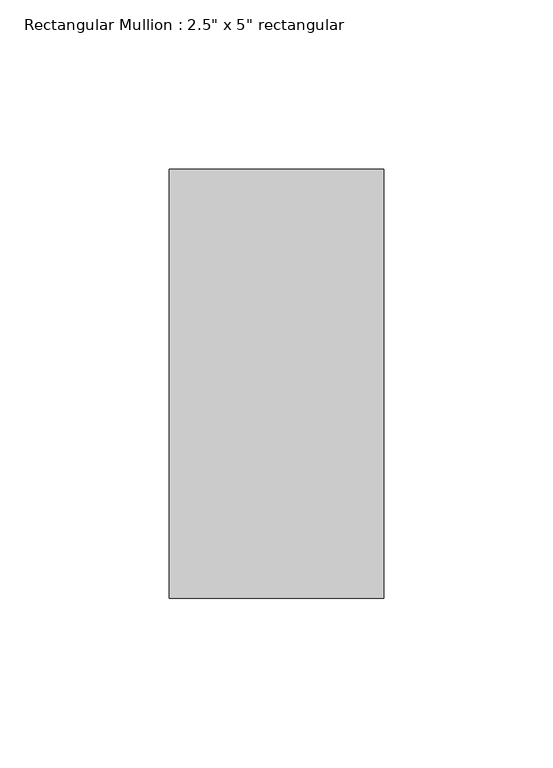
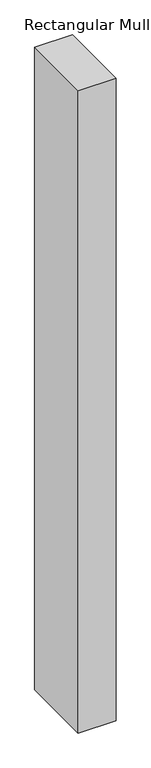
"""IFC4 building model written with IfcOpenShell, lengths in millimetres: member geometry."""

from ifc_helpers import new_model, si_unit, frame, origin, place, context, project, spatial, polyline, outline, extrude, source, transform, mapped, element, save


def member_6609bf83(model_context):
    return source(origin(), model_context, "Body", "SweptSolid", [
        extrude(outline(polyline([(0.0, 63.5), (0.0, -63.5), (-63.5, -63.5), (-63.5, 63.5), (0.0, 63.5)])), frame((0.0, 0.0, -1142.3751745), z_axis=(0.0, 0.0, 1.0), x_axis=(1.0, 0.0, 0.0)), (0.0, 0.0, 1.0), 1142.3751745),
    ])


if __name__ == "__main__":
    model = new_model("IFC4")
    model_context = context("Model", 3, world=origin())
    ifc_project = project(units=[si_unit("LENGTHUNIT", "METRE", prefix="MILLI")], contexts=[model_context])
    site = spatial("IfcSite", under=ifc_project)
    building = spatial("IfcBuilding", under=site)
    placement = place(None, origin())
    member_shape = member_6609bf83(model_context)
    element("IfcMember", 1, ObjectType="Rectangular Mullion : 2.5\" x 5\" rectangular", at=placement, inside=building, context=model_context, shape_type="MappedRepresentation", body=[
        mapped(member_shape, transform((0.0, 0.0, 0.0), x_axis=(1.0, 0.0, 0.0), y_axis=(0.0, 1.0, 0.0), z_axis=(0.0, 0.0, 1.0))),
    ])
    save(model, "model.ifc")

# Revit data of these elements
# Type "Rectangular Mullion : 2.5\" x 5\" rectangular"
#   built-in parameter 1007304 = 0.416667 (stored number, unit not read)
#   built-in parameter 1007301 = 0.104167 (stored number, unit not read)
#   built-in parameter 1007300 = 0.104167 (stored number, unit not read)
# Element 1 (IfcMember, "Rectangular Mullion : 2.5\" x 5\" rectangular")
#   Materials on its faces: "Aluminum"
# Materials
#   "Aluminum": class "Metal", colour RGB 247 247 247, transparency 0, Description = "Aluminum 6061", Cost = 0
